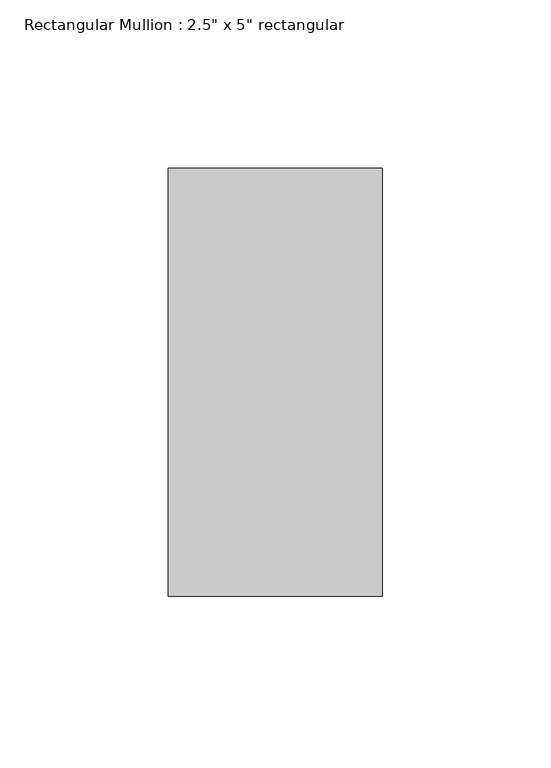
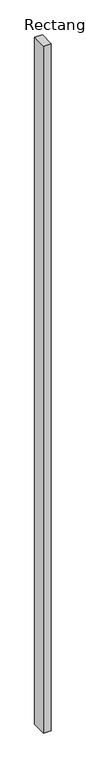
"""IFC4 building model written with IfcOpenShell, lengths in millimetres: member geometry."""

from ifc_helpers import new_model, si_unit, frame, origin, place, context, project, spatial, polyline, outline, extrude, source, transform, mapped, element, save


def member_aa97c3f9(model_context):
    return source(origin(), model_context, "Body", "SweptSolid", [
        extrude(outline(polyline([(0.0, 63.5), (0.0, -63.5), (-63.5, -63.5), (-63.5, 63.5), (0.0, 63.5)])), frame((0.0, 0.0, -6011.7116741), z_axis=(0.0, 0.0, 1.0), x_axis=(1.0, 0.0, 0.0)), (0.0, 0.0, 1.0), 6011.7116741),
    ])


if __name__ == "__main__":
    model = new_model("IFC4")
    model_context = context("Model", 3, world=origin())
    ifc_project = project(units=[si_unit("LENGTHUNIT", "METRE", prefix="MILLI")], contexts=[model_context])
    site = spatial("IfcSite", under=ifc_project)
    building = spatial("IfcBuilding", under=site)
    placement = place(None, origin())
    member_shape = member_aa97c3f9(model_context)
    element("IfcMember", 1, ObjectType="Rectangular Mullion : 2.5\" x 5\" rectangular", at=placement, inside=building, context=model_context, shape_type="MappedRepresentation", body=[
        mapped(member_shape, transform((0.0, 0.0, 0.0), x_axis=(1.0, 0.0, 0.0), y_axis=(0.0, 1.0, 0.0), z_axis=(0.0, 0.0, 1.0))),
    ])
    save(model, "model.ifc")

# Revit data of these elements
# Type "Rectangular Mullion : 2.5\" x 5\" rectangular"
#   built-in parameter 1007304 = 0.416667 (stored number, unit not read)
#   built-in parameter 1007301 = 0.104167 (stored number, unit not read)
#   built-in parameter 1007300 = 0.104167 (stored number, unit not read)
# Element 1 (IfcMember, "Rectangular Mullion : 2.5\" x 5\" rectangular")
#   Materials on its faces: "Iron, Ductile"
# Materials
#   "Iron, Ductile": class "Metal", colour RGB 0 0 0, transparency 0, Description = "Ductile cast iron", Cost = 0
